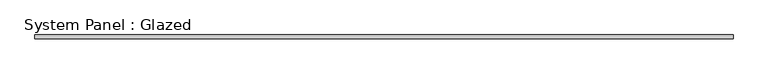
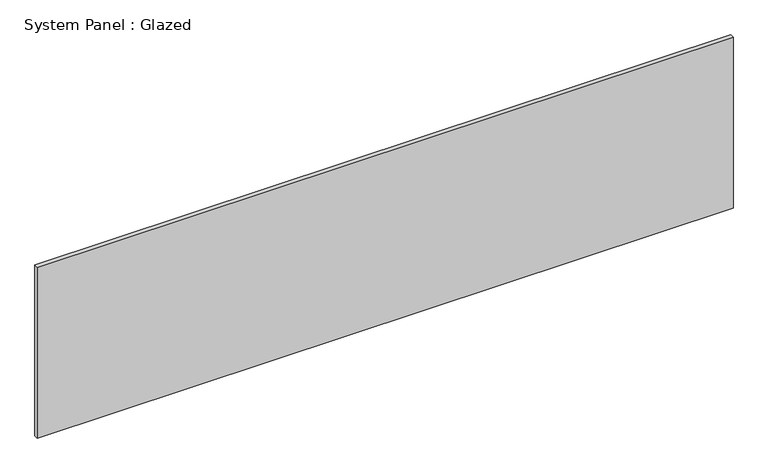
"""IFC4 building model written with IfcOpenShell, lengths in millimetres: plate geometry, System Panel : Glazed."""

from ifc_helpers import new_model, si_unit, origin, origin_with_axes, place, context, project, spatial, polyline, outline, extrude, source, transform, mapped, element, save


def system_panel_glazed_400a69f6(model_context):
    return source(origin(), model_context, "Body", "SweptSolid", [
        extrude(outline(polyline([(2346.5716886, 19.05), (-2346.5716886, 19.05), (-2346.5716886, 44.45), (2346.5716886, 44.45), (2346.5716886, 19.05)])), origin_with_axes(), (0.0, 0.0, 1.0), 1219.2),
    ])


if __name__ == "__main__":
    model = new_model("IFC4")
    model_context = context("Model", 3, world=origin())
    ifc_project = project(units=[si_unit("LENGTHUNIT", "METRE", prefix="MILLI")], contexts=[model_context])
    site = spatial("IfcSite", under=ifc_project)
    building = spatial("IfcBuilding", under=site)
    placement = place(None, origin())
    system_panel_glazed_shape = system_panel_glazed_400a69f6(model_context)
    element("IfcPlate", 1, ObjectType="System Panel : Glazed", at=placement, inside=building, context=model_context, shape_type="MappedRepresentation", body=[
        mapped(system_panel_glazed_shape, transform((0.0, 0.0, 0.0), x_axis=(1.0, 0.0, 0.0), y_axis=(0.0, 1.0, 0.0), z_axis=(0.0, 0.0, 1.0))),
    ])
    save(model, "model.ifc")

# Revit data of these elements
# Type "System Panel : Glazed"
#   Construction Type Id = "GSP4R"
#   Analytic Construction = "1/8 in Pilkington single glazing"
#   Visual Light Transmittance = 0.9
#   Solar Heat Gain Coefficient = 0.86
#   Heat Transfer Coefficient (U) = 1.18115 BTU/(h·ft²·°F)
# Element 1 (IfcPlate, "System Panel : Glazed")
#   Materials on its faces: "Glass"
# Materials
#   "Glass": class "Glass", colour RGB 0 128 192, transparency 0.75, Description = "Soda Lime Glass", Cost = 0
